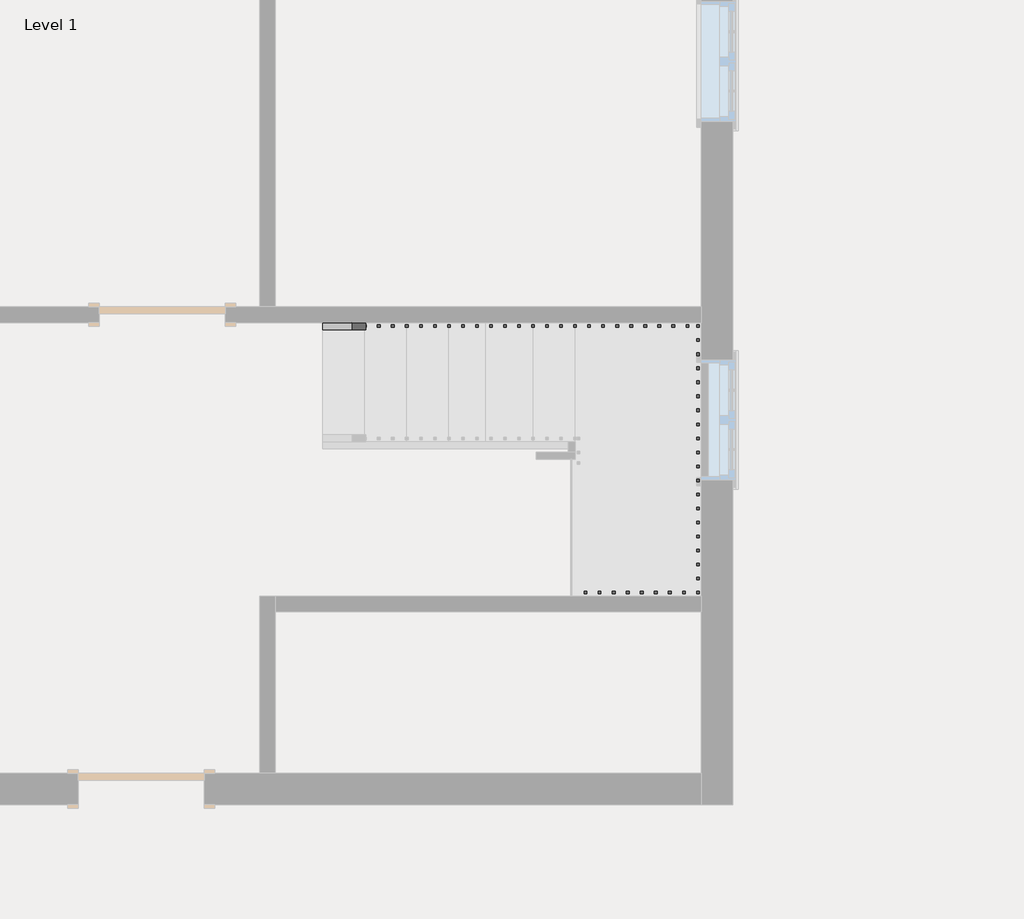
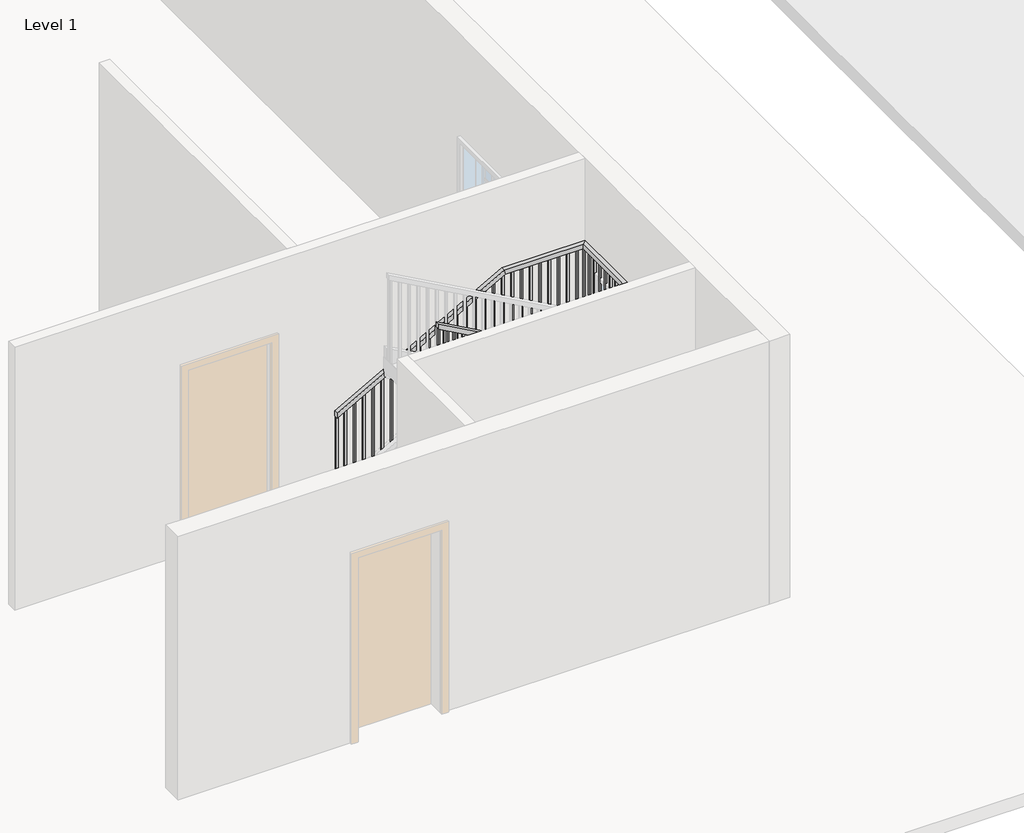
# One storey, part 2 of 3: 1 railing.
"""IFC4 building model written with IfcOpenShell, lengths in millimetres."""

from ifc_helpers import new_model, si_unit, frame, origin, place, context, project, spatial, polyline, outline, extrude, faceted_brep, element, save

model = new_model("IFC4")

# Units and contexts
model_context = context("Model", 3, world=origin())
ifc_project = project(units=[si_unit("LENGTHUNIT", "METRE", prefix="MILLI")], contexts=[model_context])

# Site, building, storey
site = spatial("IfcSite", under=ifc_project)
building = spatial("IfcBuilding", under=site)
storey = spatial("IfcBuildingStorey", under=building, Name="Level 1", Elevation=0.0)

# Railing
placement = place(None, origin())
element("IfcRailing", 1, ObjectType="Handrail - Rectangular", at=placement, inside=storey, context=model_context, shape_type="SolidModel", body=[
    faceted_brep([(-879.540747, -2065.3064015, 1083.7333333), (-879.540747, -2065.3064015, 1025.620221), (-879.540747, -2116.1064015, 1025.620221), (-879.540747, -2116.1064015, 1083.7333333), (949.259253, -2065.3064015, 2099.7333333), (962.4228552, -2065.3064015, 2048.9333333), (962.4228552, -2116.1064015, 2048.9333333), (949.259253, -2116.1064015, 2099.7333333), (1863.659253, -2065.3064015, 2099.7333333), (1863.659253, -2065.3064015, 2048.9333333), (1812.859253, -2116.1064015, 2048.9333333), (1812.859253, -2116.1064015, 2099.7333333), (1863.659253, -4046.5064015, 2099.7333333), (1863.659253, -4046.5064015, 2048.9333333), (1812.859253, -3995.7064015, 2048.9333333), (1812.859253, -3995.7064015, 2099.7333333), (1254.059253, -4046.5064015, 2099.7333333), (1240.8956508, -4046.5064015, 2048.9333333), (1240.8956508, -3995.7064015, 2048.9333333), (1254.059253, -3995.7064015, 2099.7333333), (-879.540747, -4046.5064015, 3285.0666667), (-879.540747, -3995.7064015, 3285.0666667), (-879.540747, -3995.7064015, 3226.9535543), (-879.540747, -4046.5064015, 3226.9535543)], [[[0, 1, 2, 3]], [[1, 0, 4, 5]], [[2, 1, 5, 6]], [[3, 2, 6, 7]], [[0, 3, 7, 4]], [[5, 4, 8, 9]], [[6, 5, 9, 10]], [[7, 6, 10, 11]], [[4, 7, 11, 8]], [[9, 8, 12, 13]], [[10, 9, 13, 14]], [[11, 10, 14, 15]], [[8, 11, 15, 12]], [[13, 12, 16, 17]], [[14, 13, 17, 18]], [[15, 14, 18, 19]], [[12, 15, 19, 16]], [[20, 21, 22, 23]], [[17, 16, 20, 23]], [[18, 17, 23, 22]], [[19, 18, 22, 21]], [[16, 19, 21, 20]]]),
    extrude(outline(polyline([(3189.9118876, -812.865747), (2201.3333333, -812.865747), (2201.3333333, -793.815747), (3179.3285543, -793.815747), (3189.9118876, -812.865747)])), frame((0.0, -4030.6314015, 0.0), z_axis=(0.0, 1.0, 0.0), x_axis=(0.0, 0.0, 1.0)), (0.0, 0.0, 1.0), 19.05),
    extrude(outline(polyline([(3133.4674432, -711.265747), (2201.3333333, -711.265747), (2201.3333333, -692.215747), (3122.8841099, -692.215747), (3133.4674432, -711.265747)])), frame((0.0, -4030.6314015, 0.0), z_axis=(0.0, 1.0, 0.0), x_axis=(0.0, 0.0, 1.0)), (0.0, 0.0, 1.0), 19.05),
    extrude(outline(polyline([(3077.0229988, -609.665747), (2201.3333333, -609.665747), (2201.3333333, -590.615747), (3066.4396654, -590.615747), (3077.0229988, -609.665747)])), frame((0.0, -4030.6314015, 0.0), z_axis=(0.0, 1.0, 0.0), x_axis=(0.0, 0.0, 1.0)), (0.0, 0.0, 1.0), 19.05),
    extrude(outline(polyline([(3020.5785543, -508.065747), (2032.0, -508.065747), (2032.0, -489.015747), (3009.995221, -489.015747), (3020.5785543, -508.065747)])), frame((0.0, -4030.6314015, 0.0), z_axis=(0.0, 1.0, 0.0), x_axis=(0.0, 0.0, 1.0)), (0.0, 0.0, 1.0), 19.05),
    extrude(outline(polyline([(2964.1341099, -406.465747), (2032.0, -406.465747), (2032.0, -387.415747), (2953.5507765, -387.415747), (2964.1341099, -406.465747)])), frame((0.0, -4030.6314015, 0.0), z_axis=(0.0, 1.0, 0.0), x_axis=(0.0, 0.0, 1.0)), (0.0, 0.0, 1.0), 19.05),
    extrude(outline(polyline([(2907.6896654, -304.865747), (2032.0, -304.865747), (2032.0, -285.815747), (2897.1063321, -285.815747), (2907.6896654, -304.865747)])), frame((0.0, -4030.6314015, 0.0), z_axis=(0.0, 1.0, 0.0), x_axis=(0.0, 0.0, 1.0)), (0.0, 0.0, 1.0), 19.05),
    extrude(outline(polyline([(2851.245221, -203.265747), (1862.6666667, -203.265747), (1862.6666667, -184.215747), (2840.6618876, -184.215747), (2851.245221, -203.265747)])), frame((0.0, -4030.6314015, 0.0), z_axis=(0.0, 1.0, 0.0), x_axis=(0.0, 0.0, 1.0)), (0.0, 0.0, 1.0), 19.05),
    extrude(outline(polyline([(2794.8007765, -101.665747), (1862.6666667, -101.665747), (1862.6666667, -82.615747), (2784.2174432, -82.615747), (2794.8007765, -101.665747)])), frame((0.0, -4030.6314015, 0.0), z_axis=(0.0, 1.0, 0.0), x_axis=(0.0, 0.0, 1.0)), (0.0, 0.0, 1.0), 19.05),
    extrude(outline(polyline([(2738.3563321, -0.065747), (1862.6666667, -0.065747), (1862.6666667, 18.984253), (2727.7729988, 18.984253), (2738.3563321, -0.065747)])), frame((0.0, -4030.6314015, 0.0), z_axis=(0.0, 1.0, 0.0), x_axis=(0.0, 0.0, 1.0)), (0.0, 0.0, 1.0), 19.05),
    extrude(outline(polyline([(2681.9118876, 101.534253), (1693.3333333, 101.534253), (1693.3333333, 120.584253), (2671.3285543, 120.584253), (2681.9118876, 101.534253)])), frame((0.0, -4030.6314015, 0.0), z_axis=(0.0, 1.0, 0.0), x_axis=(0.0, 0.0, 1.0)), (0.0, 0.0, 1.0), 19.05),
    extrude(outline(polyline([(2625.4674432, 203.134253), (1693.3333333, 203.134253), (1693.3333333, 222.184253), (2614.8841099, 222.184253), (2625.4674432, 203.134253)])), frame((0.0, -4030.6314015, 0.0), z_axis=(0.0, 1.0, 0.0), x_axis=(0.0, 0.0, 1.0)), (0.0, 0.0, 1.0), 19.05),
    extrude(outline(polyline([(2569.0229988, 304.734253), (1524.0, 304.734253), (1524.0, 323.784253), (2558.4396654, 323.784253), (2569.0229988, 304.734253)])), frame((0.0, -4030.6314015, 0.0), z_axis=(0.0, 1.0, 0.0), x_axis=(0.0, 0.0, 1.0)), (0.0, 0.0, 1.0), 19.05),
    extrude(outline(polyline([(2512.5785543, 406.334253), (1524.0, 406.334253), (1524.0, 425.384253), (2501.995221, 425.384253), (2512.5785543, 406.334253)])), frame((0.0, -4030.6314015, 0.0), z_axis=(0.0, 1.0, 0.0), x_axis=(0.0, 0.0, 1.0)), (0.0, 0.0, 1.0), 19.05),
    extrude(outline(polyline([(2456.1341099, 507.934253), (1524.0, 507.934253), (1524.0, 526.984253), (2445.5507765, 526.984253), (2456.1341099, 507.934253)])), frame((0.0, -4030.6314015, 0.0), z_axis=(0.0, 1.0, 0.0), x_axis=(0.0, 0.0, 1.0)), (0.0, 0.0, 1.0), 19.05),
    extrude(outline(polyline([(2399.6896654, 609.534253), (1524.0, 609.534253), (1524.0, 628.584253), (2389.1063321, 628.584253), (2399.6896654, 609.534253)])), frame((0.0, -4030.6314015, 0.0), z_axis=(0.0, 1.0, 0.0), x_axis=(0.0, 0.0, 1.0)), (0.0, 0.0, 1.0), 19.05),
    extrude(outline(polyline([(2343.245221, 711.134253), (1354.6666667, 711.134253), (1354.6666667, 730.184253), (2332.6618876, 730.184253), (2343.245221, 711.134253)])), frame((0.0, -4030.6314015, 0.0), z_axis=(0.0, 1.0, 0.0), x_axis=(0.0, 0.0, 1.0)), (0.0, 0.0, 1.0), 19.05),
    extrude(outline(polyline([(2286.8007765, 812.734253), (1354.6666667, 812.734253), (1354.6666667, 831.784253), (2276.2174432, 831.784253), (2286.8007765, 812.734253)])), frame((0.0, -4030.6314015, 0.0), z_axis=(0.0, 1.0, 0.0), x_axis=(0.0, 0.0, 1.0)), (0.0, 0.0, 1.0), 19.05),
    extrude(outline(polyline([(2230.3563321, 914.334253), (1354.6666667, 914.334253), (1354.6666667, 933.384253), (2219.7729988, 933.384253), (2230.3563321, 914.334253)])), frame((0.0, -4030.6314015, 0.0), z_axis=(0.0, 1.0, 0.0), x_axis=(0.0, 0.0, 1.0)), (0.0, 0.0, 1.0), 19.05),
    extrude(outline(polyline([(2173.9118876, 1015.934253), (1185.3333333, 1015.934253), (1185.3333333, 1034.984253), (2163.3285543, 1034.984253), (2173.9118876, 1015.934253)])), frame((0.0, -4030.6314015, 0.0), z_axis=(0.0, 1.0, 0.0), x_axis=(0.0, 0.0, 1.0)), (0.0, 0.0, 1.0), 19.05),
    extrude(outline(polyline([(2117.4674432, 1117.534253), (1185.3333333, 1117.534253), (1185.3333333, 1136.584253), (2106.8841099, 1136.584253), (2117.4674432, 1117.534253)])), frame((0.0, -4030.6314015, 0.0), z_axis=(0.0, 1.0, 0.0), x_axis=(0.0, 0.0, 1.0)), (0.0, 0.0, 1.0), 19.05),
    extrude(outline(polyline([(2061.0229988, 1219.134253), (1185.3333333, 1219.134253), (1185.3333333, 1238.184253), (2050.4396654, 1238.184253), (2061.0229988, 1219.134253)])), frame((0.0, -4030.6314015, 0.0), z_axis=(0.0, 1.0, 0.0), x_axis=(0.0, 0.0, 1.0)), (0.0, 0.0, 1.0), 19.05),
    extrude(outline(polyline([(1339.784253, -4030.6314015), (1320.734253, -4030.6314015), (1320.734253, -4011.5814015), (1339.784253, -4011.5814015), (1339.784253, -4030.6314015)])), frame((0.0, 0.0, 1185.3333333), z_axis=(0.0, 0.0, 1.0), x_axis=(1.0, 0.0, 0.0)), (0.0, 0.0, 1.0), 863.6),
    extrude(outline(polyline([(1441.384253, -4030.6314015), (1422.334253, -4030.6314015), (1422.334253, -4011.5814015), (1441.384253, -4011.5814015), (1441.384253, -4030.6314015)])), frame((0.0, 0.0, 1185.3333333), z_axis=(0.0, 0.0, 1.0), x_axis=(1.0, 0.0, 0.0)), (0.0, 0.0, 1.0), 863.6),
    extrude(outline(polyline([(1542.984253, -4030.6314015), (1523.934253, -4030.6314015), (1523.934253, -4011.5814015), (1542.984253, -4011.5814015), (1542.984253, -4030.6314015)])), frame((0.0, 0.0, 1185.3333333), z_axis=(0.0, 0.0, 1.0), x_axis=(1.0, 0.0, 0.0)), (0.0, 0.0, 1.0), 863.6),
    extrude(outline(polyline([(1644.584253, -4030.6314015), (1625.534253, -4030.6314015), (1625.534253, -4011.5814015), (1644.584253, -4011.5814015), (1644.584253, -4030.6314015)])), frame((0.0, 0.0, 1185.3333333), z_axis=(0.0, 0.0, 1.0), x_axis=(1.0, 0.0, 0.0)), (0.0, 0.0, 1.0), 863.6),
    extrude(outline(polyline([(1746.184253, -4030.6314015), (1727.134253, -4030.6314015), (1727.134253, -4011.5814015), (1746.184253, -4011.5814015), (1746.184253, -4030.6314015)])), frame((0.0, 0.0, 1185.3333333), z_axis=(0.0, 0.0, 1.0), x_axis=(1.0, 0.0, 0.0)), (0.0, 0.0, 1.0), 863.6),
    extrude(outline(polyline([(1847.784253, -3909.9814015), (1847.784253, -3929.0314015), (1828.734253, -3929.0314015), (1828.734253, -3909.9814015), (1847.784253, -3909.9814015)])), frame((0.0, 0.0, 1185.3333333), z_axis=(0.0, 0.0, 1.0), x_axis=(1.0, 0.0, 0.0)), (0.0, 0.0, 1.0), 863.6),
    extrude(outline(polyline([(1847.784253, -3808.3814015), (1847.784253, -3827.4314015), (1828.734253, -3827.4314015), (1828.734253, -3808.3814015), (1847.784253, -3808.3814015)])), frame((0.0, 0.0, 1185.3333333), z_axis=(0.0, 0.0, 1.0), x_axis=(1.0, 0.0, 0.0)), (0.0, 0.0, 1.0), 863.6),
    extrude(outline(polyline([(1847.784253, -3706.7814015), (1847.784253, -3725.8314015), (1828.734253, -3725.8314015), (1828.734253, -3706.7814015), (1847.784253, -3706.7814015)])), frame((0.0, 0.0, 1185.3333333), z_axis=(0.0, 0.0, 1.0), x_axis=(1.0, 0.0, 0.0)), (0.0, 0.0, 1.0), 863.6),
    extrude(outline(polyline([(1847.784253, -3605.1814015), (1847.784253, -3624.2314015), (1828.734253, -3624.2314015), (1828.734253, -3605.1814015), (1847.784253, -3605.1814015)])), frame((0.0, 0.0, 1185.3333333), z_axis=(0.0, 0.0, 1.0), x_axis=(1.0, 0.0, 0.0)), (0.0, 0.0, 1.0), 863.6),
    extrude(outline(polyline([(1847.784253, -3503.5814015), (1847.784253, -3522.6314015), (1828.734253, -3522.6314015), (1828.734253, -3503.5814015), (1847.784253, -3503.5814015)])), frame((0.0, 0.0, 1185.3333333), z_axis=(0.0, 0.0, 1.0), x_axis=(1.0, 0.0, 0.0)), (0.0, 0.0, 1.0), 863.6),
    extrude(outline(polyline([(1847.784253, -3401.9814015), (1847.784253, -3421.0314015), (1828.734253, -3421.0314015), (1828.734253, -3401.9814015), (1847.784253, -3401.9814015)])), frame((0.0, 0.0, 1185.3333333), z_axis=(0.0, 0.0, 1.0), x_axis=(1.0, 0.0, 0.0)), (0.0, 0.0, 1.0), 863.6),
    extrude(outline(polyline([(1847.784253, -3300.3814015), (1847.784253, -3319.4314015), (1828.734253, -3319.4314015), (1828.734253, -3300.3814015), (1847.784253, -3300.3814015)])), frame((0.0, 0.0, 1185.3333333), z_axis=(0.0, 0.0, 1.0), x_axis=(1.0, 0.0, 0.0)), (0.0, 0.0, 1.0), 863.6),
    extrude(outline(polyline([(1847.784253, -3198.7814015), (1847.784253, -3217.8314015), (1828.734253, -3217.8314015), (1828.734253, -3198.7814015), (1847.784253, -3198.7814015)])), frame((0.0, 0.0, 1185.3333333), z_axis=(0.0, 0.0, 1.0), x_axis=(1.0, 0.0, 0.0)), (0.0, 0.0, 1.0), 863.6),
    extrude(outline(polyline([(1847.784253, -3097.1814015), (1847.784253, -3116.2314015), (1828.734253, -3116.2314015), (1828.734253, -3097.1814015), (1847.784253, -3097.1814015)])), frame((0.0, 0.0, 1185.3333333), z_axis=(0.0, 0.0, 1.0), x_axis=(1.0, 0.0, 0.0)), (0.0, 0.0, 1.0), 863.6),
    extrude(outline(polyline([(1847.784253, -2995.5814015), (1847.784253, -3014.6314015), (1828.734253, -3014.6314015), (1828.734253, -2995.5814015), (1847.784253, -2995.5814015)])), frame((0.0, 0.0, 1185.3333333), z_axis=(0.0, 0.0, 1.0), x_axis=(1.0, 0.0, 0.0)), (0.0, 0.0, 1.0), 863.6),
    extrude(outline(polyline([(1847.784253, -2893.9814015), (1847.784253, -2913.0314015), (1828.734253, -2913.0314015), (1828.734253, -2893.9814015), (1847.784253, -2893.9814015)])), frame((0.0, 0.0, 1185.3333333), z_axis=(0.0, 0.0, 1.0), x_axis=(1.0, 0.0, 0.0)), (0.0, 0.0, 1.0), 863.6),
    extrude(outline(polyline([(1847.784253, -2792.3814015), (1847.784253, -2811.4314015), (1828.734253, -2811.4314015), (1828.734253, -2792.3814015), (1847.784253, -2792.3814015)])), frame((0.0, 0.0, 1185.3333333), z_axis=(0.0, 0.0, 1.0), x_axis=(1.0, 0.0, 0.0)), (0.0, 0.0, 1.0), 863.6),
    extrude(outline(polyline([(1847.784253, -2690.7814015), (1847.784253, -2709.8314015), (1828.734253, -2709.8314015), (1828.734253, -2690.7814015), (1847.784253, -2690.7814015)])), frame((0.0, 0.0, 1185.3333333), z_axis=(0.0, 0.0, 1.0), x_axis=(1.0, 0.0, 0.0)), (0.0, 0.0, 1.0), 863.6),
    extrude(outline(polyline([(1847.784253, -2589.1814015), (1847.784253, -2608.2314015), (1828.734253, -2608.2314015), (1828.734253, -2589.1814015), (1847.784253, -2589.1814015)])), frame((0.0, 0.0, 1185.3333333), z_axis=(0.0, 0.0, 1.0), x_axis=(1.0, 0.0, 0.0)), (0.0, 0.0, 1.0), 863.6),
    extrude(outline(polyline([(1847.784253, -2487.5814015), (1847.784253, -2506.6314015), (1828.734253, -2506.6314015), (1828.734253, -2487.5814015), (1847.784253, -2487.5814015)])), frame((0.0, 0.0, 1185.3333333), z_axis=(0.0, 0.0, 1.0), x_axis=(1.0, 0.0, 0.0)), (0.0, 0.0, 1.0), 863.6),
    extrude(outline(polyline([(1847.784253, -2385.9814015), (1847.784253, -2405.0314015), (1828.734253, -2405.0314015), (1828.734253, -2385.9814015), (1847.784253, -2385.9814015)])), frame((0.0, 0.0, 1185.3333333), z_axis=(0.0, 0.0, 1.0), x_axis=(1.0, 0.0, 0.0)), (0.0, 0.0, 1.0), 863.6),
    extrude(outline(polyline([(1847.784253, -2284.3814015), (1847.784253, -2303.4314015), (1828.734253, -2303.4314015), (1828.734253, -2284.3814015), (1847.784253, -2284.3814015)])), frame((0.0, 0.0, 1185.3333333), z_axis=(0.0, 0.0, 1.0), x_axis=(1.0, 0.0, 0.0)), (0.0, 0.0, 1.0), 863.6),
    extrude(outline(polyline([(1847.784253, -2182.7814015), (1847.784253, -2201.8314015), (1828.734253, -2201.8314015), (1828.734253, -2182.7814015), (1847.784253, -2182.7814015)])), frame((0.0, 0.0, 1185.3333333), z_axis=(0.0, 0.0, 1.0), x_axis=(1.0, 0.0, 0.0)), (0.0, 0.0, 1.0), 863.6),
    extrude(outline(polyline([(1752.534253, -2081.1814015), (1771.584253, -2081.1814015), (1771.584253, -2100.2314015), (1752.534253, -2100.2314015), (1752.534253, -2081.1814015)])), frame((0.0, 0.0, 1185.3333333), z_axis=(0.0, 0.0, 1.0), x_axis=(1.0, 0.0, 0.0)), (0.0, 0.0, 1.0), 863.6),
    extrude(outline(polyline([(1650.934253, -2081.1814015), (1669.984253, -2081.1814015), (1669.984253, -2100.2314015), (1650.934253, -2100.2314015), (1650.934253, -2081.1814015)])), frame((0.0, 0.0, 1185.3333333), z_axis=(0.0, 0.0, 1.0), x_axis=(1.0, 0.0, 0.0)), (0.0, 0.0, 1.0), 863.6),
    extrude(outline(polyline([(1549.334253, -2081.1814015), (1568.384253, -2081.1814015), (1568.384253, -2100.2314015), (1549.334253, -2100.2314015), (1549.334253, -2081.1814015)])), frame((0.0, 0.0, 1185.3333333), z_axis=(0.0, 0.0, 1.0), x_axis=(1.0, 0.0, 0.0)), (0.0, 0.0, 1.0), 863.6),
    extrude(outline(polyline([(1447.734253, -2081.1814015), (1466.784253, -2081.1814015), (1466.784253, -2100.2314015), (1447.734253, -2100.2314015), (1447.734253, -2081.1814015)])), frame((0.0, 0.0, 1185.3333333), z_axis=(0.0, 0.0, 1.0), x_axis=(1.0, 0.0, 0.0)), (0.0, 0.0, 1.0), 863.6),
    extrude(outline(polyline([(1346.134253, -2081.1814015), (1365.184253, -2081.1814015), (1365.184253, -2100.2314015), (1346.134253, -2100.2314015), (1346.134253, -2081.1814015)])), frame((0.0, 0.0, 1185.3333333), z_axis=(0.0, 0.0, 1.0), x_axis=(1.0, 0.0, 0.0)), (0.0, 0.0, 1.0), 863.6),
    extrude(outline(polyline([(1244.534253, -2081.1814015), (1263.584253, -2081.1814015), (1263.584253, -2100.2314015), (1244.534253, -2100.2314015), (1244.534253, -2081.1814015)])), frame((0.0, 0.0, 1185.3333333), z_axis=(0.0, 0.0, 1.0), x_axis=(1.0, 0.0, 0.0)), (0.0, 0.0, 1.0), 863.6),
    extrude(outline(polyline([(1142.934253, -2081.1814015), (1161.984253, -2081.1814015), (1161.984253, -2100.2314015), (1142.934253, -2100.2314015), (1142.934253, -2081.1814015)])), frame((0.0, 0.0, 1185.3333333), z_axis=(0.0, 0.0, 1.0), x_axis=(1.0, 0.0, 0.0)), (0.0, 0.0, 1.0), 863.6),
    extrude(outline(polyline([(1041.334253, -2081.1814015), (1060.384253, -2081.1814015), (1060.384253, -2100.2314015), (1041.334253, -2100.2314015), (1041.334253, -2081.1814015)])), frame((0.0, 0.0, 1185.3333333), z_axis=(0.0, 0.0, 1.0), x_axis=(1.0, 0.0, 0.0)), (0.0, 0.0, 1.0), 863.6),
    extrude(outline(polyline([(2036.3285543, 939.734253), (1185.3333333, 939.734253), (1185.3333333, 958.784253), (2046.9118876, 958.784253), (2036.3285543, 939.734253)])), frame((0.0, -2100.2314015, 0.0), z_axis=(0.0, 1.0, 0.0), x_axis=(0.0, 0.0, 1.0)), (0.0, 0.0, 1.0), 19.05),
    extrude(outline(polyline([(1979.8841099, 838.134253), (1016.0, 838.134253), (1016.0, 857.184253), (1990.4674432, 857.184253), (1979.8841099, 838.134253)])), frame((0.0, -2100.2314015, 0.0), z_axis=(0.0, 1.0, 0.0), x_axis=(0.0, 0.0, 1.0)), (0.0, 0.0, 1.0), 19.05),
    extrude(outline(polyline([(1923.4396654, 736.534253), (1016.0, 736.534253), (1016.0, 755.584253), (1934.0229988, 755.584253), (1923.4396654, 736.534253)])), frame((0.0, -2100.2314015, 0.0), z_axis=(0.0, 1.0, 0.0), x_axis=(0.0, 0.0, 1.0)), (0.0, 0.0, 1.0), 19.05),
    extrude(outline(polyline([(1866.995221, 634.934253), (1016.0, 634.934253), (1016.0, 653.984253), (1877.5785543, 653.984253), (1866.995221, 634.934253)])), frame((0.0, -2100.2314015, 0.0), z_axis=(0.0, 1.0, 0.0), x_axis=(0.0, 0.0, 1.0)), (0.0, 0.0, 1.0), 19.05),
    extrude(outline(polyline([(1810.5507765, 533.334253), (846.6666667, 533.334253), (846.6666667, 552.384253), (1821.1341099, 552.384253), (1810.5507765, 533.334253)])), frame((0.0, -2100.2314015, 0.0), z_axis=(0.0, 1.0, 0.0), x_axis=(0.0, 0.0, 1.0)), (0.0, 0.0, 1.0), 19.05),
    extrude(outline(polyline([(1754.1063321, 431.734253), (846.6666667, 431.734253), (846.6666667, 450.784253), (1764.6896654, 450.784253), (1754.1063321, 431.734253)])), frame((0.0, -2100.2314015, 0.0), z_axis=(0.0, 1.0, 0.0), x_axis=(0.0, 0.0, 1.0)), (0.0, 0.0, 1.0), 19.05),
    extrude(outline(polyline([(1697.6618876, 330.134253), (846.6666667, 330.134253), (846.6666667, 349.184253), (1708.245221, 349.184253), (1697.6618876, 330.134253)])), frame((0.0, -2100.2314015, 0.0), z_axis=(0.0, 1.0, 0.0), x_axis=(0.0, 0.0, 1.0)), (0.0, 0.0, 1.0), 19.05),
    extrude(outline(polyline([(1641.2174432, 228.534253), (677.3333333, 228.534253), (677.3333333, 247.584253), (1651.8007765, 247.584253), (1641.2174432, 228.534253)])), frame((0.0, -2100.2314015, 0.0), z_axis=(0.0, 1.0, 0.0), x_axis=(0.0, 0.0, 1.0)), (0.0, 0.0, 1.0), 19.05),
    extrude(outline(polyline([(1584.7729988, 126.934253), (677.3333333, 126.934253), (677.3333333, 145.984253), (1595.3563321, 145.984253), (1584.7729988, 126.934253)])), frame((0.0, -2100.2314015, 0.0), z_axis=(0.0, 1.0, 0.0), x_axis=(0.0, 0.0, 1.0)), (0.0, 0.0, 1.0), 19.05),
    extrude(outline(polyline([(1528.3285543, 25.334253), (677.3333333, 25.334253), (677.3333333, 44.384253), (1538.9118876, 44.384253), (1528.3285543, 25.334253)])), frame((0.0, -2100.2314015, 0.0), z_axis=(0.0, 1.0, 0.0), x_axis=(0.0, 0.0, 1.0)), (0.0, 0.0, 1.0), 19.05),
    extrude(outline(polyline([(1471.8841099, -76.265747), (508.0, -76.265747), (508.0, -57.215747), (1482.4674432, -57.215747), (1471.8841099, -76.265747)])), frame((0.0, -2100.2314015, 0.0), z_axis=(0.0, 1.0, 0.0), x_axis=(0.0, 0.0, 1.0)), (0.0, 0.0, 1.0), 19.05),
    extrude(outline(polyline([(1415.4396654, -177.865747), (508.0, -177.865747), (508.0, -158.815747), (1426.0229988, -158.815747), (1415.4396654, -177.865747)])), frame((0.0, -2100.2314015, 0.0), z_axis=(0.0, 1.0, 0.0), x_axis=(0.0, 0.0, 1.0)), (0.0, 0.0, 1.0), 19.05),
    extrude(outline(polyline([(1358.995221, -279.465747), (508.0, -279.465747), (508.0, -260.415747), (1369.5785543, -260.415747), (1358.995221, -279.465747)])), frame((0.0, -2100.2314015, 0.0), z_axis=(0.0, 1.0, 0.0), x_axis=(0.0, 0.0, 1.0)), (0.0, 0.0, 1.0), 19.05),
    extrude(outline(polyline([(1302.5507765, -381.065747), (338.6666667, -381.065747), (338.6666667, -362.015747), (1313.1341099, -362.015747), (1302.5507765, -381.065747)])), frame((0.0, -2100.2314015, 0.0), z_axis=(0.0, 1.0, 0.0), x_axis=(0.0, 0.0, 1.0)), (0.0, 0.0, 1.0), 19.05),
    extrude(outline(polyline([(1246.1063321, -482.665747), (338.6666667, -482.665747), (338.6666667, -463.615747), (1256.6896654, -463.615747), (1246.1063321, -482.665747)])), frame((0.0, -2100.2314015, 0.0), z_axis=(0.0, 1.0, 0.0), x_axis=(0.0, 0.0, 1.0)), (0.0, 0.0, 1.0), 19.05),
    extrude(outline(polyline([(1189.6618876, -584.265747), (338.6666667, -584.265747), (338.6666667, -565.215747), (1200.245221, -565.215747), (1189.6618876, -584.265747)])), frame((0.0, -2100.2314015, 0.0), z_axis=(0.0, 1.0, 0.0), x_axis=(0.0, 0.0, 1.0)), (0.0, 0.0, 1.0), 19.05),
    extrude(outline(polyline([(1133.2174432, -685.865747), (169.3333333, -685.865747), (169.3333333, -666.815747), (1143.8007765, -666.815747), (1133.2174432, -685.865747)])), frame((0.0, -2100.2314015, 0.0), z_axis=(0.0, 1.0, 0.0), x_axis=(0.0, 0.0, 1.0)), (0.0, 0.0, 1.0), 19.05),
    extrude(outline(polyline([(1076.7729988, -787.465747), (169.3333333, -787.465747), (169.3333333, -768.415747), (1087.3563321, -768.415747), (1076.7729988, -787.465747)])), frame((0.0, -2100.2314015, 0.0), z_axis=(0.0, 1.0, 0.0), x_axis=(0.0, 0.0, 1.0)), (0.0, 0.0, 1.0), 19.05),
    extrude(outline(polyline([(1847.784253, -4011.5814015), (1847.784253, -4030.6314015), (1828.734253, -4030.6314015), (1828.734253, -4011.5814015), (1847.784253, -4011.5814015)])), frame((0.0, 0.0, 1185.3333333), z_axis=(0.0, 0.0, 1.0), x_axis=(1.0, 0.0, 0.0)), (0.0, 0.0, 1.0), 863.6),
    extrude(outline(polyline([(1828.734253, -2081.1814015), (1847.784253, -2081.1814015), (1847.784253, -2100.2314015), (1828.734253, -2100.2314015), (1828.734253, -2081.1814015)])), frame((0.0, 0.0, 1185.3333333), z_axis=(0.0, 0.0, 1.0), x_axis=(1.0, 0.0, 0.0)), (0.0, 0.0, 1.0), 863.6),
    extrude(outline(polyline([(3226.9535543, -879.540747), (2201.3333333, -879.540747), (2201.3333333, -860.490747), (3216.370221, -860.490747), (3226.9535543, -879.540747)])), frame((0.0, -4030.6314015, 0.0), z_axis=(0.0, 1.0, 0.0), x_axis=(0.0, 0.0, 1.0)), (0.0, 0.0, 1.0), 19.05),
    extrude(outline(polyline([(1025.620221, -879.540747), (169.3333333, -879.540747), (169.3333333, -860.490747), (1036.2035543, -860.490747), (1025.620221, -879.540747)])), frame((0.0, -2100.2314015, 0.0), z_axis=(0.0, 1.0, 0.0), x_axis=(0.0, 0.0, 1.0)), (0.0, 0.0, 1.0), 19.05),
])

save(model, "model.ifc")

# Revit data of these elements
# Type "Handrail - Rectangular"
#   Assembly Code = "C2010400"
#   built-in parameter 1008612 = 0.0416667 (stored number, unit not read)
#   built-in parameter 1008611 = 0.0416667 (stored number, unit not read)
#   built-in parameter 1008609 = 0.333333 (stored number, unit not read)
#   built-in parameter 1008604 = 0.166667 (stored number, unit not read)
#   built-in parameter 1008603 = 0.166667 (stored number, unit not read)
#   Railing Height = 3' - 0"
#   built-in parameter 1008630 = 2
#   built-in parameter 1008610 = 2
#   built-in parameter 1008618 = Baluster - Square : 3/4"
# Element 1 (IfcRailing, "Handrail - Rectangular")
#   Phase Created = New Construction
